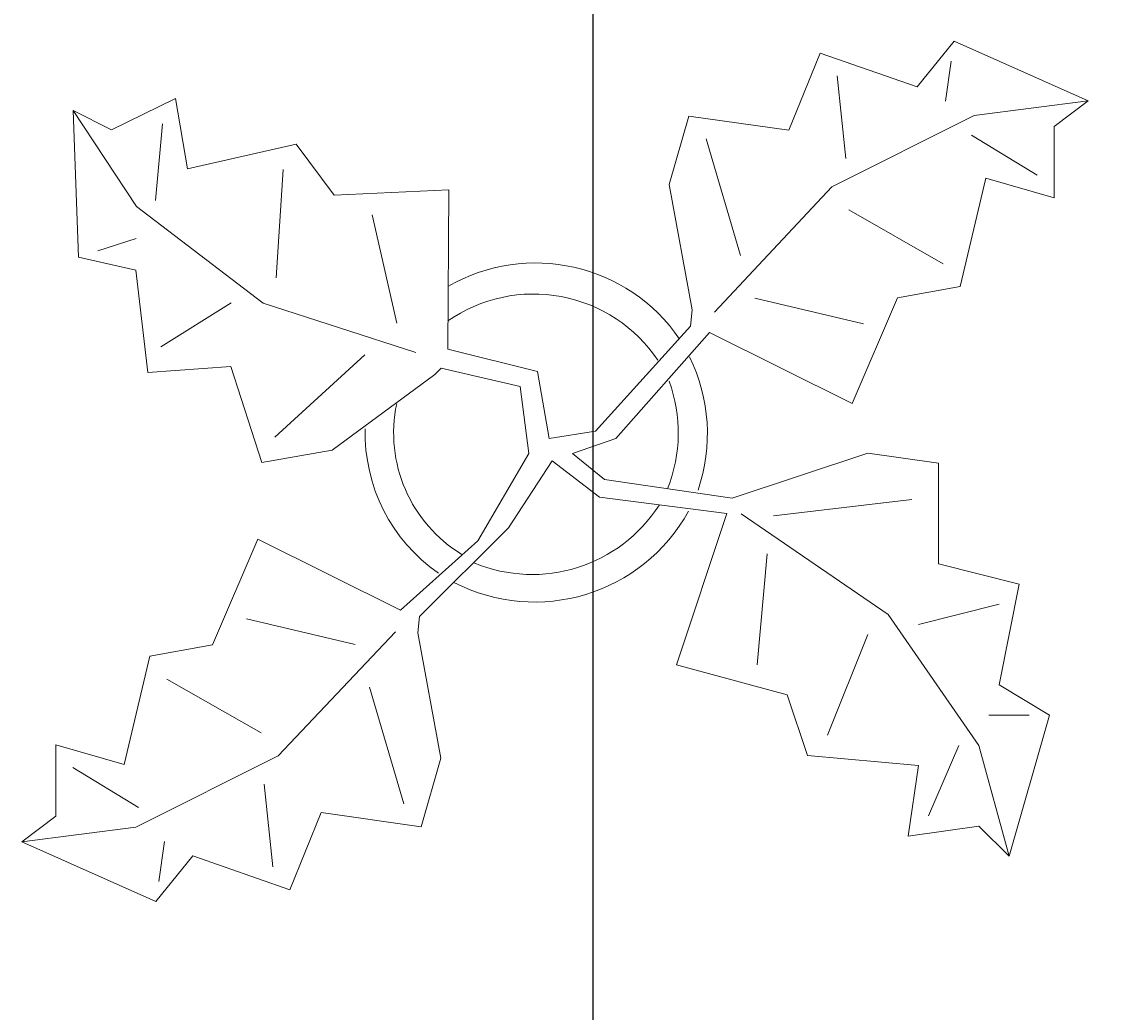
# Model space of a CAD drawing. Units: inches. Extents: x -301 to 715, y -607 to 364.
# Tile 58 of 141: x -136 to -111, y -260 to -237. Entities that reach past the tile are written whole.
import ezdxf

# ---------------------------------------------------------------- set-up
doc = ezdxf.new("R2010")
doc.units = ezdxf.units.IN
doc.header["$MEASUREMENT"] = 0
doc.layers.add('A-ANNO-DIMS', color=2, linetype='Continuous', lineweight=18)
doc.layers.add('L-PLNT', color=94, linetype='Continuous', lineweight=13)
doc.styles.get("Standard").update_dxf_attribs({"font": 'arial.ttf'})
doc.dimstyles.get("Standard").update_dxf_attribs({"dimtxt": 0.18, "dimasz": 0.18, "dimexe": 0.18, "dimexo": 0.0625, "dimgap": 0.09, "dimtad": 0, "dimtih": 1, "dimtoh": 1, "dimdec": 1, "dimzin": 0, "dimdsep": 46, "dimlunit": 4, "dimtxsty": 'Standard', "dimcen": 0.09, "dimclrd": 3, "dimclre": 4, "dimclrt": 6, "dimadec": 0, "dimazin": 0, "dimtfac": 1, "dimtdec": 1, "dimtofl": 0, "dimtmove": 0, "dimatfit": 3, "dimfxl": 1, "dimtfill": 2, "dimtfillclr": 51, "dimtolj": 1, "dimtzin": 0, "dimarcsym": 0})

# ---------------------------------------------------------------- blocks, each defined once
blk = doc.blocks.new('Plant - Rubber or Philodendron')
for p, q in [((13.3837, 12.301), (14.68, 13.9039)), ((14.68, 13.9039), (19.3848, 11.8146)), ((8.8871, 10.7908), (9.9809, 13.4933)), ((9.9809, 13.4933), (13.3837, 12.301)), ((14.5816, 13.2037), (14.3848, 11.8033)), ((10.5828, 12.6946), (10.8893, 9.7953)), ((-14.8639, 10.7964), (-12.6195, 11.8975)), ((-12.6195, 11.8975), (-12.1909, 9.4345)), ((-16.2005, 11.4774), (-13.9899, 8.1064)), ((-16.2005, 11.4774), (-14.8639, 10.7964)), ((-16.0159, 6.3329), (-16.2005, 11.4774)), ((19.3848, 11.8146), (15.3859, 11.3055)), ((19.3848, 11.8146), (18.1868, 10.9119)), ((4.6914, 8.8812), (5.3859, 11.2828)), ((5.3859, 11.2828), (8.8871, 10.7908)), ((15.3859, 11.3055), (10.3916, 8.7942)), ((-13.3174, 8.325), (-13.0735, 11.0065)), ((18.1868, 10.9119), (18.1925, 8.4119)), ((5.9878, 10.4842), (7.1971, 6.3869)), ((15.2875, 10.6053), (17.5907, 9.2105)), ((-12.1909, 9.4345), (-8.3829, 10.3)), ((-8.3829, 10.3), (-7.0549, 8.501)), ((-8.8369, 9.409), (-9.0894, 5.6095)), ((4.6914, 8.8812), (5.5014, 4.4831)), ((10.3916, 8.7942), (6.2847, 4.4028)), ((15.7909, 9.1065), (14.8995, 5.3044)), ((18.1925, 8.4119), (15.7909, 9.1065)), ((-7.0549, 8.501), (-3.0284, 8.6941)), ((-3.0284, 8.6941), (-3.0709, 3.1041)), ((-13.9899, 8.1064), (-9.5434, 4.7185)), ((-4.8529, 4.012), (-5.7184, 7.82)), ((14.2977, 6.1031), (10.9934, 7.9956)), ((-15.3434, 6.5514), (-13.9984, 6.9884)), ((-14.0069, 5.8704), (-16.0159, 6.3329)), ((-13.5868, 2.2894), (-14.0069, 5.8704)), ((14.8995, 5.3044), (12.7005, 4.8994)), ((-13.1329, 3.1804), (-10.6614, 4.727)), ((-9.5434, 4.7185), (-4.1917, 2.9888)), ((7.7005, 4.8881), (11.5025, 3.9967)), ((12.7005, 4.8994), (11.1089, 1.1958)), ((5.4346, 3.9146), (5.5014, 4.4831)), ((2.1141, 0.2298), (5.4346, 3.9146)), ((6.1032, 3.6844), (2.8262, -0.031)), ((11.1089, 1.1958), (6.1032, 3.6844)), ((-3.0709, 3.1041), (0.0797, 2.3163)), ((-9.1318, 0.0195), (-5.9793, 2.9025)), ((-10.6784, 2.491), (-13.5868, 2.2894)), ((-9.5858, -0.8715), (-10.6784, 2.491)), ((-3.5248, 2.2131), (-3.3011, 2.4355)), ((-3.3011, 2.4355), (-0.5306, 1.7947)), ((0.0797, 2.3163), (0.4866, -0.031)), ((-7.1228, -0.443), (-3.5248, 2.2131)), ((-0.5306, 1.7947), (-0.2255, -0.5527)), ((-0.5306, 1.7947), (-0.5306, 1.7947)), ((0.4866, -0.031), (2.1141, 0.2298)), ((2.8262, -0.031), (1.3003, -0.5527)), ((-7.1228, -0.443), (-9.5858, -0.8715)), ((-2.019, -3.6148), (-0.2255, -0.5527)), ((1.3003, -0.5527), (2.4193, -1.4655)), ((11.6605, -0.5413), (6.895, -2.1175)), ((11.6605, -0.5413), (14.1354, -0.8948)), ((-0.9375, -3.1608), (0.5883, -0.8135)), ((0.5883, -0.8135), (2.2447, -2.0916)), ((14.1354, -0.8948), (14.1354, -4.4304)), ((2.4193, -1.4655), (6.895, -2.1175)), ((2.2447, -2.0916), (6.7108, -2.6626)), ((8.3544, -2.7453), (13.1973, -2.1704)), ((4.943, -7.9659), (6.7108, -2.6626)), ((12.3677, -6.1981), (7.219, -2.6772)), ((-4.0579, -6.2781), (-0.9375, -3.1608)), ((-11.3237, -7.2629), (-9.7321, -3.5593)), ((-9.7321, -3.5593), (-4.7264, -6.0479)), ((-2.019, -3.6148), (-4.7264, -6.0479)), ((8.125, -4.0768), (7.7715, -7.9659)), ((14.1354, -4.4304), (16.9638, -5.1375)), ((16.9638, -5.1375), (16.2567, -8.673)), ((16.2567, -5.8446), (13.4283, -6.5517)), ((-6.3237, -7.2516), (-10.1257, -6.3602)), ((-4.1246, -6.8466), (-4.0579, -6.2781)), ((15.5496, -10.7943), (12.3677, -6.1981)), ((-9.0148, -11.1577), (-4.9047, -6.8122)), ((-3.3146, -11.2447), (-4.1246, -6.8466)), ((10.2463, -10.4408), (11.6605, -6.9053)), ((-13.5228, -7.6679), (-11.3237, -7.2629)), ((-14.4141, -11.4699), (-13.5228, -7.6679)), ((8.8321, -9.0266), (4.943, -7.9659)), ((-12.921, -8.4665), (-9.6166, -10.359)), ((-4.611, -12.8477), (-5.8203, -8.7504)), ((16.2567, -8.673), (18.0245, -9.7337)), ((9.5392, -11.1479), (8.8321, -9.0266)), ((17.3174, -9.7337), (15.9032, -9.7337)), ((18.0245, -9.7337), (16.6103, -14.6834)), ((-16.8157, -10.7754), (-14.4141, -11.4699)), ((-16.8101, -13.2754), (-16.8157, -10.7754)), ((14.8425, -10.7943), (13.7819, -13.2692)), ((16.6103, -14.6834), (15.5496, -10.7943)), ((-14.0091, -13.669), (-9.0148, -11.1577)), ((-3.3146, -11.2447), (-4.0092, -13.6463)), ((13.4283, -11.5015), (9.5392, -11.1479)), ((-13.9107, -12.9688), (-16.2139, -11.574)), ((13.0748, -13.9763), (13.4283, -11.5015)), ((-9.206, -15.0581), (-9.5126, -12.1588)), ((-18.008, -14.1781), (-16.8101, -13.2754)), ((-7.5103, -13.1543), (-8.6042, -15.8568)), ((-4.0092, -13.6463), (-7.5103, -13.1543)), ((-18.008, -14.1781), (-14.0091, -13.669)), ((15.5496, -13.6228), (13.0748, -13.9763)), ((16.6103, -14.6834), (15.5496, -13.6228)), ((-13.3032, -16.2674), (-18.008, -14.1781)), ((-13.2048, -15.5672), (-13.008, -14.1668)), ((-12.0069, -14.6645), (-13.3032, -16.2674)), ((-8.6042, -15.8568), (-12.0069, -14.6645))]:
    blk.add_line(p, q)
for centre, radius, start, end in [((0, 0), 6.1275, 34.37569, 120.1028), ((-0.0601, -0.2075), 5.2461, 33.82192, 124.9414), ((-0.098, 0.1364), 6.1288, 341.2017, 26.09184), ((-0.2664, 0.1682), 5.2775, 338.4094, 20.03007), ((0.0308, 0.1664), 5, 168.1647, 238.6725), ((0.0308, 0.1664), 6, 178.6147, 235.1169), ((-0.0234, 0.3825), 6.1492, 242.5812, 331.2714), ((-0.1102, 0.4886), 5.2883, 247.3711, 327.472)]:
    blk.add_arc(centre, radius, start, end)
blk = doc.blocks.new('*D158')
at = {"layer": 'A-ANNO-DIMS', "color": 4, "lineweight": -2, "transparency": 16777216}
for p, q in [((-122.603, 221.62), (-122.603, -296.865)), ((-50.603, 221.62), (-50.603, -296.865))]:
    blk.add_line(p, q, dxfattribs=at)
at = {"layer": 'A-ANNO-DIMS', "color": 3, "lineweight": -2, "transparency": 16777216}
for p, q in [((-122.423, -296.685), (-86.933, -296.685)), ((-50.783, -296.685), (-86.274, -296.685))]:
    blk.add_line(p, q, dxfattribs=at)
at = {"layer": 'A-ANNO-DIMS', "color": 3, "transparency": 16777216}
for points in [[(-122.423, -296.655), (-122.423, -296.715), (-122.603, -296.685)], [(-50.783, -296.655), (-50.783, -296.715), (-50.603, -296.685)]]:
    blk.add_solid(points, dxfattribs=at)
at = {"layer": 'Defpoints', "color": 0, "transparency": 16777216}
for p in [(-122.603, 221.682), (-50.603, 221.682), (-50.603, -296.685)]:
    blk.add_point(p, dxfattribs=at)
at = {"layer": 'A-ANNO-DIMS', "color": 6, "transparency": 16777216, "insert": (-86.603, -296.685), "char_height": 0.18, "attachment_point": 5, "bg_fill": 1, "box_fill_scale": 1.25, "bg_fill_color": 51, "bg_fill_transparency": 0}
blk.add_mtext('\\A1;6\'-0"', dxfattribs=at)

msp = doc.modelspace()

# ---------------------------------------------------------------- block references
at = {"layer": 'L-PLNT', "xscale": 0.6613521884636907, "yscale": 0.6613521884636907, "zscale": 0.6613521884636907}
msp.add_blockref('Plant - Rubber or Philodendron', (-123.938, -246.796), dxfattribs=at)

# ---------------------------------------------------------------- dimensions: what is measured, and where the dimension line sits
at = {"layer": 'A-ANNO-DIMS'}
dim = msp.add_linear_dim(base=(-50.603, -296.685), p1=(-122.603, 221.682), p2=(-50.603, 221.682), dimstyle='Standard', override={"dimdec": 1, "dimlfac": 1, "dimrnd": 0, "dimzin": 1, "dimdsep": 46, "dimlunit": 4, "dimfrac": 2}, dxfattribs=at)
dim.commit()
dim.dimension.update_dxf_attribs({"geometry": '*D158', "text_midpoint": (-86.603, -296.685)})

doc.saveas('drawing.dxf')
